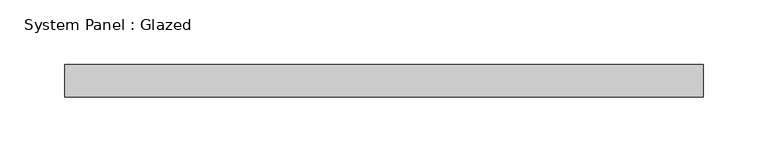
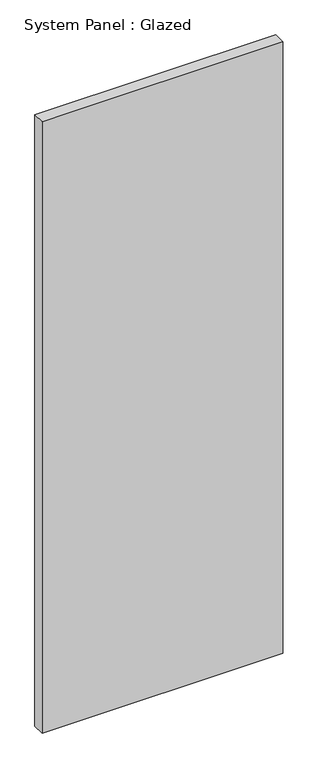
"""IFC4 building model written with IfcOpenShell, lengths in millimetres: plate geometry, System Panel : Glazed."""

from ifc_helpers import new_model, si_unit, origin, origin_with_axes, place, context, project, spatial, polyline, outline, extrude, source, transform, mapped, element, save


def system_panel_glazed_1cd5f074(model_context):
    return source(origin(), model_context, "Body", "SweptSolid", [
        extrude(outline(polyline([(247.65, 19.05), (-247.65, 19.05), (-247.65, 44.45), (247.65, 44.45), (247.65, 19.05)])), origin_with_axes(), (0.0, 0.0, 1.0), 1330.6985165),
    ])


if __name__ == "__main__":
    model = new_model("IFC4")
    model_context = context("Model", 3, world=origin())
    ifc_project = project(units=[si_unit("LENGTHUNIT", "METRE", prefix="MILLI")], contexts=[model_context])
    site = spatial("IfcSite", under=ifc_project)
    building = spatial("IfcBuilding", under=site)
    placement = place(None, origin())
    system_panel_glazed_shape = system_panel_glazed_1cd5f074(model_context)
    element("IfcPlate", 1, ObjectType="System Panel : Glazed", at=placement, inside=building, context=model_context, shape_type="MappedRepresentation", body=[
        mapped(system_panel_glazed_shape, transform((0.0, 0.0, 0.0), x_axis=(1.0, 0.0, 0.0), y_axis=(0.0, 1.0, 0.0), z_axis=(0.0, 0.0, 1.0))),
    ])
    save(model, "model.ifc")

# Revit data of these elements
# Type "System Panel : Glazed"
#   Construction Type Id = "GSP4R"
#   Analytic Construction = "1/8 in Pilkington single glazing"
#   Visual Light Transmittance = 0.9
#   Solar Heat Gain Coefficient = 0.86
#   Heat Transfer Coefficient (U) = 1.18115 BTU/(h·ft²·°F)
#   Define Thermal Properties by = 1
# Element 1 (IfcPlate, "System Panel : Glazed")
#   Materials on its faces: "Glass"
# Materials
#   "Glass": class "Glass", colour RGB 0 128 192, transparency 0.75, Description = "Soda Lime Glass", Cost = 0
